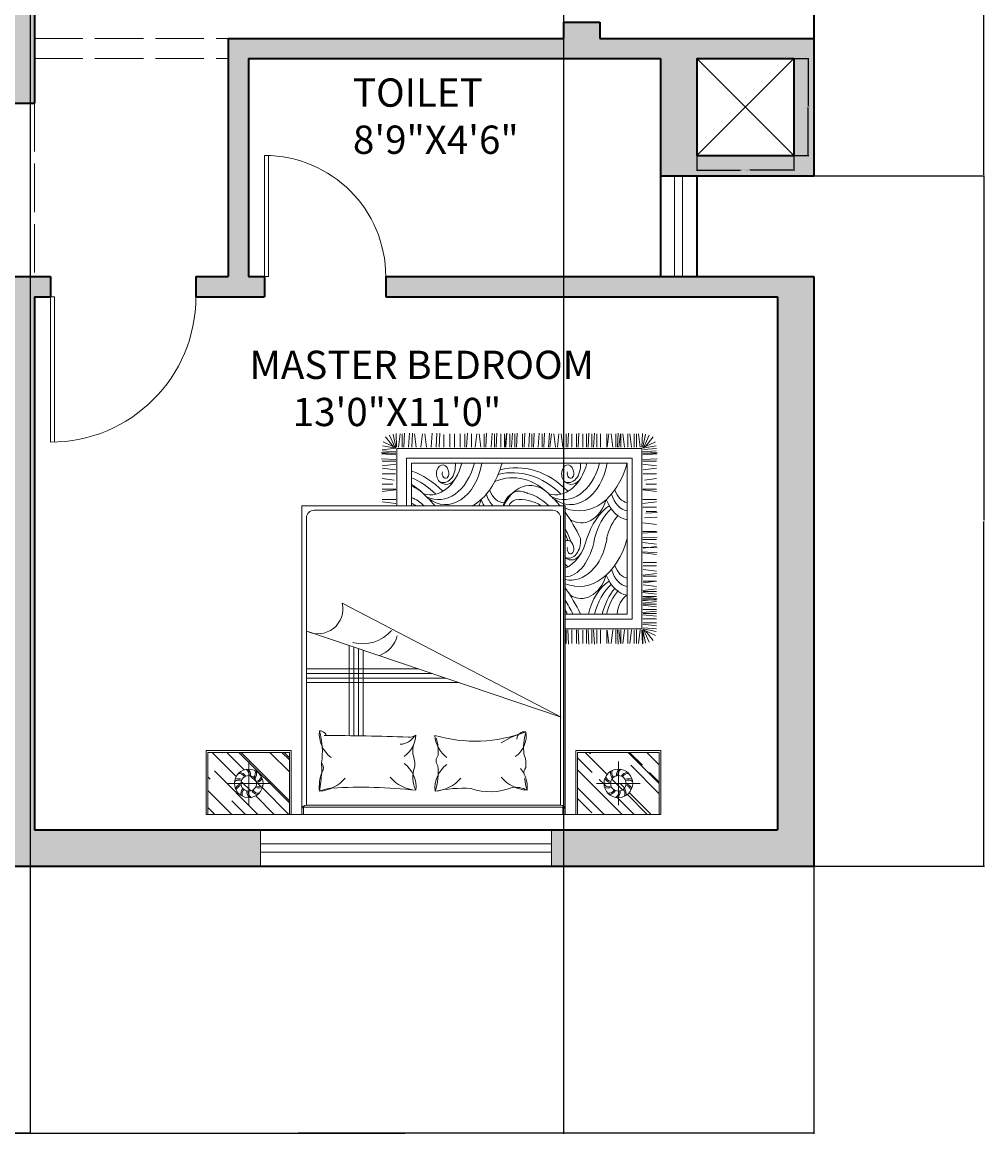
# Model space of a CAD drawing. Units: inches. Extents: x 2540 to 3167, y 3083 to 4007.
# Tile 7 of 15: x 2929 to 3167, y 3083 to 3359. Entities that reach past the tile are written whole.
import ezdxf

# ---------------------------------------------------------------- set-up
doc = ezdxf.new("R2010")
doc.units = ezdxf.units.IN
doc.linetypes.add('ACAD_ISO02W100', pattern=[15, 12, -3])
for name, color, linetype, lineweight in [('A-ANNO-DIMS', 2, 'Continuous', 18), ('A-AREA-IDEN', 7, 'Continuous', 18), ('A-DOOR', 4, 'Continuous', 18), ('A-FLOR-OPEN', 8, 'Continuous', 13), ('A-FURN', 8, 'Continuous', 13), ('A-GLAZ', 4, 'Continuous', 18)]:
    doc.layers.add(name, color=color, linetype=linetype, lineweight=lineweight)
for name, color, linetype, lineweight, true_color in [('A-WALL', 143, 'Continuous', 35, 0x7aafdf), ('A-WALL-OVHD', 143, 'ACAD_ISO02W100', 18, 0x7aafdf), ('A-WALL-PATT', 143, 'Continuous', 13, 0x7aafdf)]:
    doc.layers.add(name, color=color, linetype=linetype, lineweight=lineweight, true_color=true_color)
doc.styles.get("Standard").update_dxf_attribs({"font": 'arial.ttf'})
doc.dimstyles.get("Standard").update_dxf_attribs({"dimtxt": 0.18, "dimasz": 0.18, "dimexe": 0.18, "dimexo": 0.0625, "dimgap": 0.09, "dimtad": 0, "dimtih": 1, "dimtoh": 1, "dimdec": 4, "dimzin": 0, "dimdsep": 46, "dimtxsty": 'Standard', "dimcen": 0.09, "dimadec": 0, "dimazin": 0, "dimtfac": 1, "dimtdec": 4, "dimtofl": 0, "dimtmove": 0, "dimatfit": 3, "dimfxl": 1, "dimtolj": 1, "dimtzin": 0, "dimarcsym": 0})

# ---------------------------------------------------------------- blocks, each defined once
blk = doc.blocks.new('A$C64B41DC1')
for p, q in [((0, 2.5079), (2.9903, 2.5079)), ((0, 2.0879), (0, 2.5079)), ((0.012, 2.4618), (0.0581, 2.5079)), ((0.012, 2.3515), (0.1684, 2.5079)), ((0.012, 2.0999), (0.012, 2.5079)), ((0.0543, 2.2213), (0.3409, 2.5079)), ((0.1689, 2.4179), (0.2589, 2.5079)), ((0.3265, 2.386), (0.4484, 2.5079)), ((0.3699, 2.3332), (0.5445, 2.5079)), ((0.548, 2.5079), (0.548, 2.0999)), ((0.56, 2.5079), (0.56, 2.0879)), ((0.6301, 2.5079), (0.6301, 0.4779)), ((0.6401, 2.461), (0.6401, 2.5079)), ((0.6401, 2.5079), (2.344, 2.5079)), ((2.344, 2.5079), (2.3601, 2.5079)), ((2.344, 2.5079), (2.344, 2.461)), ((2.3601, 2.5079), (2.3601, 2.4761)), ((2.3601, 0.4779), (2.3601, 2.5079)), ((2.4303, 2.5079), (2.4303, 2.0879)), ((2.4423, 2.5079), (2.4423, 2.0999)), ((2.4423, 2.3333), (2.6169, 2.5079)), ((2.4423, 2.2145), (2.7357, 2.5079)), ((2.4423, 2.404), (2.5354, 2.4971)), ((2.705, 2.398), (2.8149, 2.5079)), ((2.7691, 2.3772), (2.8998, 2.5079)), ((2.7819, 2.3646), (2.9252, 2.5079)), ((2.9783, 2.0999), (2.9783, 2.5079)), ((2.9903, 2.0879), (2.9903, 2.5079)), ((0.2157, 2.0999), (0.548, 2.4322)), ((0.2299, 2.0999), (0.548, 2.418)), ((0.2804, 2.1597), (0.2804, 2.4481)), ((2.344, 2.461), (0.6401, 2.461)), ((0.6601, 2.4461), (1.4951, 2.4461)), ((0.6601, 2.4461), (0.6601, 0.5579)), ((1.4951, 2.4461), (0.6697, 2.4461)), ((2.3301, 2.4461), (1.4951, 2.4461)), ((2.3301, 0.5579), (2.3301, 2.4461)), ((2.7099, 2.1597), (2.7099, 2.4481)), ((0.2311, 2.2906), (0.2937, 2.3532)), ((2.6674, 2.2756), (2.7382, 2.3464)), ((2.7914, 2.1846), (2.9783, 2.3715)), ((0.012, 2.261), (0.0275, 2.2765)), ((0.1362, 2.3039), (0.4246, 2.3039)), ((0.2905, 2.2539), (0.3304, 2.2938)), ((0.3405, 2.3039), (0.3605, 2.3238)), ((2.8541, 2.3039), (2.5657, 2.3039)), ((2.5849, 2.2779), (2.6158, 2.3088)), ((2.6158, 2.3088), (2.6313, 2.3243)), ((2.7249, 2.3076), (2.7512, 2.3339)), ((2.7746, 2.0999), (2.9783, 2.3036)), ((2.9144, 2.2312), (2.9783, 2.2951)), ((0.0404, 2.0999), (0.1982, 2.2578)), ((0.1365, 2.0999), (0.251, 2.2144)), ((0.4194, 2.0999), (0.548, 2.2285)), ((2.4423, 2.1353), (2.5382, 2.2312)), ((2.4918, 2.0999), (2.6366, 2.2447)), ((0.4986, 2.0999), (0.548, 2.1493)), ((0.5127, 2.0999), (0.548, 2.1352)), ((2.7831, 2.0999), (2.8678, 2.1846)), ((2.8962, 2.0999), (2.9783, 2.182)), ((0.56, 2.0879), (0, 2.0879)), ((0.548, 2.0999), (0.012, 2.0999)), ((2.4303, 2.0879), (2.9903, 2.0879)), ((2.4423, 2.0999), (2.9783, 2.0999)), ((2.5172, 2.0999), (2.5269, 2.1096)), ((0.9415, 1.9902), (0.9415, 1.3975)), ((0.9715, 1.9906), (0.9715, 1.4076)), ((1.0015, 1.991), (1.0015, 1.4177)), ((1.0315, 1.9916), (1.0315, 1.4279)), ((2.3349, 1.8678), (0.6613, 1.3029)), ((0.8956, 1.1191), (2.3349, 1.8678)), ((1.6636, 1.6412), (0.6601, 1.6412)), ((1.5748, 1.6112), (0.6601, 1.6112)), ((2.377, 1.295), (2.3822, 1.3891)), ((2.4451, 1.295), (2.4503, 1.3891)), ((2.5105, 1.295), (2.5157, 1.3891)), ((2.5471, 1.295), (2.5524, 1.3891)), ((2.7043, 1.295), (2.7095, 1.3891)), ((2.3665, 1.295), (2.3665, 1.3839)), ((2.4032, 1.295), (2.4032, 1.3839)), ((2.4346, 1.295), (2.4346, 1.3839)), ((2.4774, 1.2957), (2.4774, 1.3837)), ((2.5, 1.295), (2.5, 1.3839)), ((2.5367, 1.295), (2.5367, 1.3839)), ((2.5681, 1.295), (2.5681, 1.3839)), ((2.5918, 1.295), (2.5918, 1.3839)), ((2.6346, 1.2957), (2.6346, 1.3837)), ((2.6362, 1.2957), (2.6467, 1.3839)), ((2.6729, 1.295), (2.6624, 1.3839)), ((2.6938, 1.295), (2.6938, 1.3839)), ((2.7127, 1.2957), (2.7232, 1.3839)), ((2.7253, 1.295), (2.7253, 1.3839)), ((2.7494, 1.295), (2.7389, 1.3839)), ((2.7718, 1.295), (2.7718, 1.3839)), ((2.7959, 1.295), (2.7854, 1.3839)), ((2.8146, 1.2957), (2.8146, 1.3837)), ((2.8146, 1.2957), (2.8146, 1.3837)), ((2.8282, 1.295), (2.8282, 1.3839)), ((2.8282, 1.295), (2.8282, 1.3839)), ((2.8523, 1.295), (2.8418, 1.3839)), ((2.8523, 1.295), (2.8418, 1.3839)), ((2.8653, 1.2966), (2.8688, 1.3861)), ((2.8711, 1.2957), (2.8711, 1.3837)), ((2.8711, 1.2957), (2.8875, 1.3822)), ((2.8713, 1.2927), (2.954, 1.3315)), ((2.8765, 1.2958), (2.9132, 1.3758)), ((2.8893, 1.3011), (2.9394, 1.3636)), ((2.3601, 1.2873), (2.8639, 1.2873)), ((2.8639, 1.2873), (2.8639, 0.1018)), ((2.8716, 1.2565), (2.9605, 1.2669)), ((2.8717, 1.2884), (2.9588, 1.3058)), ((2.8723, 1.2489), (2.9603, 1.2489)), ((2.8744, 1.2817), (2.9603, 1.2869)), ((2.3601, 1.2233), (2.7999, 1.2233)), ((2.3601, 1.1913), (2.7679, 1.1912)), ((2.7679, 1.1912), (2.7679, 0.1978)), ((2.7999, 1.2233), (2.7999, 0.1658)), ((2.8716, 1.2212), (2.9605, 1.2212)), ((2.8716, 1.1947), (2.9605, 1.2052)), ((2.8716, 1.181), (2.9605, 1.1705)), ((2.8723, 1.1872), (2.9603, 1.1872)), ((2.8716, 1.1595), (2.9605, 1.1595)), ((2.8716, 1.133), (2.9605, 1.1435)), ((2.8716, 1.1193), (2.9605, 1.1088)), ((2.8716, 1.1035), (2.9605, 1.093)), ((2.8716, 1.0965), (2.9605, 1.0965)), ((2.8723, 1.1255), (2.9603, 1.1255)), ((2.8716, 1.086), (2.9657, 1.0913)), ((2.8716, 1.0756), (2.9605, 1.0756)), ((2.8716, 1.0491), (2.9605, 1.0596)), ((2.8716, 1.0354), (2.9605, 1.0249)), ((2.8723, 1.0858), (2.9605, 1.0753)), ((2.8723, 1.0416), (2.9603, 1.0416)), ((2.8723, 0.9987), (2.9605, 1.0092)), ((2.8723, 0.985), (2.9605, 0.9745)), ((2.8723, 0.9735), (2.9603, 0.9735)), ((2.8716, 0.9346), (2.9605, 0.9241)), ((2.8723, 0.9408), (2.9603, 0.9408)), ((2.8723, 0.8979), (2.9605, 0.9084)), ((2.8723, 0.8726), (2.9603, 0.8726)), ((2.8723, 0.8505), (2.9603, 0.8505)), ((2.8716, 0.7885), (2.9605, 0.799)), ((2.8716, 0.7818), (2.9657, 0.787)), ((2.8716, 0.7503), (2.9657, 0.7556)), ((2.8716, 0.7204), (2.9605, 0.7309)), ((2.8723, 0.7571), (2.9605, 0.7466)), ((2.8716, 0.6995), (2.9605, 0.6995)), ((2.8716, 0.689), (2.9657, 0.6838)), ((2.8716, 0.6576), (2.9657, 0.6523)), ((2.8716, 0.6471), (2.9605, 0.6471)), ((2.8716, 0.5903), (2.9605, 0.6007)), ((2.882, 0.5582), (2.9657, 0.5536)), ((2.8909, 0.5263), (2.9657, 0.5222)), ((2.8928, 0.5169), (2.9605, 0.5169)), ((0.6301, 0.4779), (2.3601, 0.4779)), ((0.7101, 0.5079), (2.2801, 0.5079)), ((1.2465, 0.4625), (1.1576, 0.452)), ((1.2542, 0.1018), (1.2542, 0.4779)), ((1.3182, 0.1658), (1.3182, 0.4779)), ((1.3502, 0.1978), (1.3502, 0.4779)), ((2.8716, 0.4877), (2.9603, 0.4877)), ((2.8716, 0.4625), (2.9605, 0.452)), ((1.2465, 0.3746), (1.1576, 0.3851)), ((1.2465, 0.4365), (1.1577, 0.4365)), ((1.2465, 0.3684), (1.1577, 0.3684)), ((2.8716, 0.4365), (2.9603, 0.4365)), ((2.8716, 0.3746), (2.9605, 0.3851)), ((2.8716, 0.3684), (2.9603, 0.3684)), ((1.2355, 0.3092), (1.1576, 0.3)), ((1.2285, 0.3357), (1.1577, 0.3357)), ((2.8826, 0.3092), (2.9605, 0.3)), ((2.8896, 0.3357), (2.9603, 0.3357)), ((1.2457, 0.2423), (1.1576, 0.2319)), ((1.2457, 0.2676), (1.1577, 0.2676)), ((2.8723, 0.2676), (2.9603, 0.2676)), ((2.8723, 0.2423), (2.9605, 0.2319)), ((1.2465, 0.1742), (1.1524, 0.169)), ((1.2465, 0.2057), (1.1576, 0.2161)), ((1.2465, 0.1847), (1.1576, 0.1847)), ((2.7999, 0.1658), (1.3182, 0.1658)), ((2.7679, 0.1978), (1.3502, 0.1978)), ((2.8716, 0.2057), (2.9605, 0.2161)), ((2.8716, 0.1847), (2.9605, 0.1847)), ((2.8716, 0.1742), (2.9657, 0.169)), ((1.2465, 0.1428), (1.1524, 0.1376)), ((1.2465, 0.1334), (1.1524, 0.1281)), ((1.2465, 0.1323), (1.1576, 0.1323)), ((1.2465, 0.1323), (1.1576, 0.1323)), ((1.2465, 0.1), (1.1576, 0.1105)), ((1.2465, 0.1229), (1.1588, 0.1168)), ((1.2464, 0.1007), (1.1592, 0.0833)), ((1.2468, 0.0964), (1.1641, 0.0576)), ((1.2288, 0.088), (1.1787, 0.0255)), ((1.2415, 0.0933), (1.2049, 0.0133)), ((1.247, 0.0934), (1.2306, 0.0069)), ((1.2527, 0.0925), (1.2493, 0.003)), ((2.8639, 0.1018), (1.2542, 0.1018)), ((1.2658, 0.0941), (1.2762, 0.0052)), ((1.2899, 0.0941), (1.2899, 0.0052)), ((1.2999, 0.0941), (1.3051, 0)), ((1.3313, 0.0941), (1.3365, 0)), ((1.3523, 0.0941), (1.3575, 0)), ((1.3804, 0.0941), (1.3699, 0.0052)), ((1.4119, 0.0934), (1.4223, 0.0052)), ((1.4485, 0.0941), (1.438, 0.0052)), ((1.48, 0.0941), (1.4852, 0)), ((1.5114, 0.0941), (1.5166, 0)), ((1.5323, 0.0941), (1.5376, 0)), ((1.5638, 0.0941), (1.5638, 0.0105)), ((1.6021, 0.0941), (1.6021, 0.0052)), ((1.6336, 0.0941), (1.6336, 0.0052)), ((1.6702, 0.0941), (1.6702, 0.0052)), ((1.7017, 0.0941), (1.7017, 0.0052)), ((1.7122, 0.0941), (1.7174, 0)), ((1.7445, 0.0934), (1.7445, 0.0054)), ((1.7698, 0.0934), (1.7803, 0.0052)), ((1.8065, 0.0941), (1.796, 0.0052)), ((1.8274, 0.0941), (1.8274, 0.0052)), ((1.8379, 0.0941), (1.8431, 0)), ((1.8746, 0.0941), (1.8798, 0)), ((1.8955, 0.0941), (1.8955, 0.0052)), ((1.906, 0.0941), (1.9113, 0)), ((1.9384, 0.0934), (1.9384, 0.0054)), ((1.9609, 0.0941), (1.9609, 0.0052)), ((1.9636, 0.0934), (1.9741, 0.0052)), ((1.9714, 0.0941), (1.9766, 0)), ((1.9976, 0.0941), (1.9976, 0.0052)), ((2.0081, 0.0941), (2.0133, 0)), ((2.029, 0.0941), (2.029, 0.0052)), ((2.0395, 0.0941), (2.0447, 0)), ((2.0797, 0.0941), (2.0797, 0.0052)), ((2.0902, 0.0941), (2.0954, 0)), ((2.1216, 0.0941), (2.1269, 0)), ((2.1412, 0.0941), (2.1412, 0.0052)), ((2.1517, 0.0941), (2.1569, 0)), ((2.1831, 0.0941), (2.1884, 0)), ((2.2093, 0.0941), (2.2093, 0.0052)), ((2.2198, 0.0941), (2.225, 0)), ((2.2512, 0.0941), (2.2565, 0)), ((2.2603, 0.0934), (2.2707, 0.0052)), ((2.2969, 0.0941), (2.2864, 0.0052)), ((2.3089, 0.0934), (2.3193, 0.0052)), ((2.3455, 0.0941), (2.3351, 0.0052)), ((2.3665, 0.0941), (2.3665, 0.0052)), ((2.377, 0.0941), (2.3822, 0)), ((2.4032, 0.0941), (2.4032, 0.0052)), ((2.4346, 0.0941), (2.4346, 0.0052)), ((2.4451, 0.0941), (2.4503, 0)), ((2.4774, 0.0934), (2.4774, 0.0054)), ((2.5, 0.0941), (2.5, 0.0052)), ((2.5105, 0.0941), (2.5157, 0)), ((2.5367, 0.0941), (2.5367, 0.0052)), ((2.5471, 0.0941), (2.5524, 0)), ((2.5681, 0.0941), (2.5681, 0.0052)), ((2.5918, 0.0941), (2.5918, 0.0052)), ((2.6346, 0.0934), (2.6346, 0.0054)), ((2.6362, 0.0934), (2.6467, 0.0052)), ((2.6729, 0.0941), (2.6624, 0.0052)), ((2.6938, 0.0941), (2.6938, 0.0052)), ((2.7043, 0.0941), (2.7095, 0)), ((2.7127, 0.0934), (2.7232, 0.0052)), ((2.7253, 0.0941), (2.7253, 0.0052)), ((2.7494, 0.0941), (2.7389, 0.0052)), ((2.7718, 0.0941), (2.7718, 0.0052)), ((2.7959, 0.0941), (2.7854, 0.0052)), ((2.8146, 0.0934), (2.8146, 0.0054)), ((2.8282, 0.0941), (2.8282, 0.0052)), ((2.8523, 0.0941), (2.8418, 0.0052)), ((2.8653, 0.0925), (2.8688, 0.003)), ((2.8711, 0.0934), (2.8875, 0.0069)), ((2.8713, 0.0964), (2.954, 0.0576)), ((2.8716, 0.1428), (2.9657, 0.1376)), ((2.8716, 0.1334), (2.9657, 0.1281)), ((2.8716, 0.1323), (2.9605, 0.1323)), ((2.8716, 0.1229), (2.9593, 0.1168)), ((2.8717, 0.1007), (2.9588, 0.0833)), ((2.8744, 0.1074), (2.9603, 0.1022)), ((2.8765, 0.0933), (2.9132, 0.0133)), ((2.8893, 0.088), (2.9394, 0.0255))]:
    blk.add_line(p, q)
at = {"ltscale": 10}
for p, q in [((1.4859, 1.5812), (0.6601, 1.5812)), ((1.397, 1.5512), (0.6601, 1.5512))]:
    blk.add_line(p, q, dxfattribs=at)
for centre, radius in [((0.2804, 2.3039), 0.0942), ((0.2804, 2.3039), 0.051), ((2.7099, 2.3039), 0.0942), ((2.7099, 2.3039), 0.051)]:
    blk.add_circle(centre, radius)
for centre, radius, start, end in [((0.6601, 2.4761), 0.03, 180, 270), ((2.3301, 2.4761), 0.03, 270, 0), ((0.2417, 2.3614), 0.0462, 196.30017, 256.53802), ((0.2887, 2.3745), 0.0605, 172.17003, 218.48975), ((0.2828, 2.3731), 0.0462, 160.30017, 220.53802), ((0.3286, 2.3561), 0.0605, 136.17003, 182.48975), ((0.3231, 2.3585), 0.0462, 124.30017, 184.53802), ((0.3501, 2.3178), 0.0605, 100.17003, 146.48975), ((0.347, 2.323), 0.0462, 88.30017, 148.53802), ((1.0526, 2.3302), 0.3085, 175.30484, 198.69419), ((-0.8702, 2.0941), 1.6364, 4.80985, 9.18918), ((0.8579, 2.6278), 0.2948, 247.51785, 264.26696), ((0.728, 2.111), 0.245, 40.4189, 85.9871), ((1.0164, 5.7096), 3.3803, 266.81337, 276.16021), ((1.3963, 2.1044), 0.245, 94.0129, 139.5811), ((1.1858, 2.3288), 0.1943, 306.5711, 5.88998), ((1.5348, 2.2652), 0.1767, 151.77364, 201.69827), ((1.6986, 2.3355), 0.1943, 174.11002, 233.4289), ((1.1481, 2.2311), 0.3783, 353.49469, 19.18669), ((1.6871, 3.192), 0.8561, 257.74383, 273.62843), ((1.4882, 2.111), 0.245, 40.4189, 85.9871), ((1.8674, 1.9709), 0.3878, 68.20259, 108.9817), ((2.1269, 2.1044), 0.245, 94.0129, 139.5811), ((2.0342, 2.4856), 0.1563, 261.59582, 298.90918), ((1.9165, 2.3288), 0.1943, 333.73715, 5.88998), ((2.6058, 2.2028), 0.517, 163.60457, 172.3273), ((2.6433, 2.323), 0.0462, 31.46198, 91.69983), ((2.6402, 2.3178), 0.0605, 33.51025, 79.82997), ((2.6672, 2.3585), 0.0462, 355.46198, 55.69983), ((2.6617, 2.3561), 0.0605, 357.51025, 43.82997), ((2.7075, 2.3731), 0.0462, 319.46198, 19.69983), ((2.7016, 2.3745), 0.0605, 321.51025, 7.82997), ((2.7486, 2.3614), 0.0462, 283.46198, 343.69983), ((0.2153, 2.3276), 0.0462, 232.30017, 292.53802), ((0.2158, 2.3336), 0.0605, 244.17003, 290.48975), ((0.2457, 2.3659), 0.0605, 208.17003, 254.48975), ((0.272, 2.2333), 0.0605, 352.17003, 38.48975), ((0.3449, 2.2742), 0.0605, 64.17003, 110.48975), ((0.3455, 2.2802), 0.0462, 52.30017, 112.53802), ((0.3191, 2.2464), 0.0462, 16.30017, 76.53802), ((0.3151, 2.2419), 0.0605, 28.17003, 74.48975), ((2.6448, 2.2802), 0.0462, 67.46198, 127.69983), ((2.6454, 2.2742), 0.0605, 69.51025, 115.82997), ((2.6752, 2.2419), 0.0605, 105.51025, 151.82997), ((2.6712, 2.2464), 0.0462, 103.46198, 163.69983), ((2.7182, 2.2333), 0.0605, 141.51025, 187.82997), ((2.7744, 2.3336), 0.0605, 249.51025, 295.82997), ((2.775, 2.3276), 0.0462, 247.46198, 307.69983), ((2.7446, 2.3659), 0.0605, 285.51025, 331.82997), ((0.2138, 2.2848), 0.0462, 268.30017, 328.53802), ((0.2107, 2.29), 0.0605, 280.17003, 326.48975), ((0.2377, 2.2493), 0.0462, 304.30017, 4.53802), ((0.2322, 2.2517), 0.0605, 316.17003, 2.48975), ((0.2779, 2.2347), 0.0462, 340.30017, 40.53802), ((0.7274, 2.2013), 0.0446, 314.4736, 42.17134), ((-1.6008, 2.277), 2.3618, 357.39054, 358.88764), ((1.204, 2.1778), 0.1681, 337.01697, 7.53676), ((1.9165, 2.3288), 0.1943, 320.94042, 333.73715), ((2.1347, 2.2313), 0.0459, 165.35061, 223.26844), ((1.9346, 2.1778), 0.1681, 337.01697, 7.53676), ((2.7123, 2.2347), 0.0462, 139.46198, 199.69983), ((2.7581, 2.2517), 0.0605, 177.51025, 223.82997), ((2.7526, 2.2493), 0.0462, 175.46198, 235.69983), ((2.7796, 2.29), 0.0605, 213.51025, 259.82997), ((2.7765, 2.2848), 0.0462, 211.46198, 271.69983), ((0.9385, 1.978), 0.1943, 126.5711, 185.88998), ((0.2688, 2.0945), 0.4956, 344.0243, 8.70709), ((1.1858, 1.9714), 0.1943, 4.31813, 53.4289), ((1.7059, 1.9714), 0.204, 127.11975, 175.09005), ((1.5671, 2.1546), 0.0547, 142.08329, 220.902), ((1.9394, 1.991), 0.1651, 351.26213, 55.75721), ((1.2687, 1.9248), 0.1223, 33.62799, 86.47438), ((1.5415, 2.0969), 0.1834, 175.22328, 196.23004), ((1.1965, 2.0983), 0.3299, 343.79543, 3.55541), ((2.4617, 2.0719), 0.3745, 173.82958, 196.4356), ((0.7417, 2.0149), 0.057, 273.47085, 328.54118), ((0.7246, 18.8439), 16.8552, 270.17399, 272.05214), ((1.3401, 1.9404), 0.0603, 49.09906, 101.37023), ((1.7676, 1.0629), 0.9631, 69.65065, 105.96307), ((2.2748, 2.5795), 0.6373, 238.34989, 254.31375), ((2.0911, 2.0123), 0.0478, 179.77267, 283.80184), ((0.728, 2.2025), 0.245, 274.0129, 278.34166), ((1.0747, 1.2871), 0.1871, 14.1863, 69.12121), ((0.7347, 1.1553), 0.1649, 347.31088, 116.44537), ((1.0274, 1.1334), 0.2527, 40.62904, 104.37123), ((0.7101, 0.5579), 0.05, 180, 270), ((2.2801, 0.5579), 0.05, 270, 0)]:
    blk.add_arc(centre, radius, start, end)
for centre, major_axis, ratio, start_param, end_param in [((1.9938, 1.6262), (0, -0.7531), 0.68, 0.797284, 0.954936), ((2.0643, 1.466), (0, -0.5322), 0.68, 7.239912, 7.311536), ((1.9052, 1.7397), (0, -0.9842), 0.68, 0.74745, 0.979724), ((2.7455, 1.3081), (0, 0.3614), 0.68, 1.900046, 2.742661), ((2.7868, 1.3081), (0, 0.3614), 0.68, 1.900046, 2.614747), ((2.8372, 1.3081), (0, 0.3614), 0.68, 1.900046, 2.479658), ((2.8607, 1.3211), (0, 0.3614), 0.68, 1.938265, 2.479658), ((2.8057, 1.2079), (0, -0.1524), 0.68, 4.821745, 5.895886), ((2.4665, 0.8216), (0, -0.2664), 0.68, 2.006169, 3.565187), ((2.4513, 0.5069), (0, 0.502), 0.68, 5.095327, 6.553458), ((2.7862, 0.8069), (0, -0.2615), 0.68, 3.244645, 4.205018), ((2.396, 0.6032), (0, 0.3641), 0.68, -1.3172, 0.145284), ((2.7784, 0.8289), (0, -0.1802), 0.68, 3.227058, 4.318474), ((2.7821, 0.7971), (0, -0.1589), 0.68, 3.272942, 4.229533), ((2.3507, 0.5642), (0.0073, 0.3819), 0.56205, -1.21172, -0.009991), ((2.2964, 0.5771), (0, -0.3263), 0.68, 1.938944, 2.850232), ((2.0403, 1.6015), (0, -0.8763), 0.68, 6.849801, 6.887077), ((2.4005, 0.7132), (0, -0.1214), 0.68, 2.284368, 3.652258), ((2.3834, 0.7081), (0, 0.1147), 0.68, 4.593909, 6.585576), ((2.3774, 0.7653), (0, -0.0593), 0.68, 5.841311, 7.755362), ((2.3961, 0.7628), (0, -0.0317), 0.68, 1.462497, 5.046281), ((1.9938, 1.1295), (-0.0678, 0.7439), 0.610498, 3.917146, 4.063997), ((2.0643, 0.9693), (0, -0.5322), 0.68, 7.239912, 7.336618), ((1.9052, 1.243), (0, -0.9842), 0.68, 0.74745, 0.979724), ((2.7455, 0.8114), (-0.0599, 0.3735), 0.695517, 1.775813, 2.548612), ((2.7868, 0.8114), (0, 0.3614), 0.68, 1.900046, 2.614747), ((2.8607, 0.8243), (0, 0.3614), 0.68, 1.938265, 2.479658), ((2.4665, 0.3249), (0, -0.2664), 0.68, 2.006169, 3.565187), ((2.4513, 0.0102), (0, 0.502), 0.68, 5.095327, 6.553458), ((2.7862, 0.3102), (0, -0.2615), 0.68, 3.244645, 4.205018), ((2.7784, 0.3322), (0, -0.1802), 0.68, 3.227058, 4.318474), ((1.242, 0.9693), (0, -0.5322), 0.68, 6.586764, 6.677612), ((1.1714, 1.1295), (-0.1157, 0.7241), 0.59432, 3.291697, 3.50733), ((1.0828, 1.243), (0, -0.9842), 0.68, 0.565948, 0.680366), ((1.5283, 0.0674), (0, -0.3703), 0.68, 1.930561, 3.464283), ((1.5736, 0.1065), (0, 0.3641), 0.68, -1.3172, 0.476403), ((1.6289, 0.0102), (0, 0.502), 0.68, 6.655152, 6.661293), ((1.6289, 0.0102), (0, 0.502), 0.68, 5.095327, 5.911219), ((1.6442, 0.3249), (0, -0.2664), 0.68, 2.006169, 2.182797), ((1.9638, 0.3102), (0, -0.2615), 0.68, 4.015924, 4.205018), ((1.956, 0.3322), (0, -0.1802), 0.68, 3.770744, 4.318474), ((1.9597, 0.3004), (0, -0.1589), 0.68, 3.14258, 4.229533), ((2.0606, 0.5616), (0, -0.1803), 0.68, 5.194792, 5.929328), ((2.0606, 0.5616), (0, -0.1803), 0.68, 5.194792, 6.723255), ((2.1315, 0.6603), (0, -0.3155), 0.68, 5.328638, 6.949396), ((2.0549, 0.5656), (0, -0.1303), 0.68, 5.450951, 6.054641), ((2.0643, 0.9693), (0, -0.5322), 0.68, 6.20013, 6.677612), ((1.9938, 1.1295), (-0.0678, 0.7439), 0.610498, 3.199135, 3.592282), ((1.9052, 1.243), (0, -0.9842), 0.68, 0.565948, 0.680366), ((2.3507, 0.0674), (0, -0.3703), 0.68, 1.930561, 3.464283), ((2.396, 0.1065), (0, 0.3641), 0.68, -1.3172, 0.476403), ((2.4513, 0.0102), (0, 0.502), 0.68, 6.655152, 6.661293), ((2.7821, 0.3004), (0, -0.1589), 0.68, 3.272942, 4.229533), ((1.1933, 0.9181), (0, -0.624), 0.68, 0.378672, 0.625379), ((1.3091, 0.6603), (0, -0.3155), 0.68, 6.475719, 6.949396), ((1.1911, 1.1066), (0, 0.8458), 0.68, 3.421828, 3.728616), ((1.2179, 1.1047), (0, -0.8763), 0.68, 6.507006, 6.887077), ((1.474, 0.0804), (0, -0.3263), 0.68, 1.938944, 3.339184), ((2.0157, 0.9181), (0, -0.624), 0.68, -0.280078, 0.625379), ((2.0135, 1.1066), (0, 0.8458), 0.68, 2.978727, 3.728616), ((2.0403, 1.1047), (0, -0.8763), 0.68, 6.099302, 6.887077), ((2.2964, 0.0804), (0, -0.3263), 0.68, 1.938944, 3.339184), ((1.555, 0.2685), (0, -0.0593), 0.68, 3.732151, 7.755362), ((1.5781, 0.2165), (0, -0.1214), 0.68, 2.284368, 3.726131), ((1.561, 0.2114), (0, 0.1147), 0.68, 4.593909, 6.647252), ((1.5737, 0.2661), (0, -0.0317), 0.68, 1.462497, 5.046281), ((2.3774, 0.2685), (0, -0.0593), 0.68, 3.732151, 7.755362), ((2.4005, 0.2165), (0, -0.1214), 0.68, 2.284368, 3.726131), ((2.3834, 0.2114), (0, 0.1147), 0.68, 4.593909, 6.647252), ((2.3961, 0.2661), (0, -0.0317), 0.68, 1.462497, 5.046281)]:
    blk.add_ellipse(centre, major_axis=major_axis, ratio=ratio, start_param=start_param, end_param=end_param)
blk = doc.blocks.new('DOOR-SWING-36IN')
for p, q in [((36, 0), (0, 0)), ((36, 1), (0.01, 1)), ((36, 1), (36, 0))]:
    blk.add_line(p, q)
blk.add_arc((36, 0), 36, 90, 180)
blk = doc.blocks.new('DOOR-SWING-30IN')
for p, q in [((0, 0), (0, 30)), ((1, 0), (1, 29.98)), ((0, 0), (1, 0))]:
    blk.add_line(p, q)
blk.add_arc((0, 0), 30, 0, 90)
blk = doc.blocks.new('WIN-72IN')
for p, q in [((9, 72), (0, 72)), ((3.5, 0), (3.5, 72)), ((5.5, 0), (5.5, 72)), ((9, 0), (0, 0))]:
    blk.add_line(p, q)
blk = doc.blocks.new('OPENING-CROSS-24IN')
for p, q in [((24, 24), (0, 0)), ((0, 24), (24, 0))]:
    blk.add_line(p, q)
blk = doc.blocks.new('*D41')
at = {"layer": 'A-ANNO-DIMS', "color": 0, "lineweight": -2, "transparency": 16777216}
for p, q in [((3095.51, 3325.65), (3095.51, 3321.93)), ((3119.51, 3325.65), (3119.51, 3321.93)), ((3095.69, 3322.11), (3106.37, 3322.11)), ((3119.33, 3322.11), (3108.65, 3322.11))]:
    blk.add_line(p, q, dxfattribs=at)
at = {"layer": 'A-ANNO-DIMS', "color": 0, "transparency": 16777216}
for points in [[(3095.69, 3322.14), (3095.69, 3322.08), (3095.51, 3322.11)], [(3119.33, 3322.14), (3119.33, 3322.08), (3119.51, 3322.11)]]:
    blk.add_solid(points, dxfattribs=at)
at = {"layer": 'Defpoints', "color": 0, "transparency": 16777216}
for p in [(3095.51, 3325.71), (3119.51, 3325.71), (3119.51, 3322.11)]:
    blk.add_point(p, dxfattribs=at)
at = {"layer": 'A-ANNO-DIMS', "color": 0, "transparency": 16777216, "insert": (3107.51, 3322.11), "char_height": 0.18, "attachment_point": 5}
blk.add_mtext('\\A1;OPENING 24 TYP.', dxfattribs=at)
blk = doc.blocks.new('*D42')
at = {"layer": 'A-ANNO-DIMS', "color": 0, "lineweight": -2, "transparency": 16777216}
for p, q in [((3119.57, 3349.71), (3123.29, 3349.71)), ((3123.11, 3349.53), (3123.11, 3337.89)), ((3123.11, 3325.89), (3123.11, 3337.53)), ((3119.57, 3325.71), (3123.29, 3325.71))]:
    blk.add_line(p, q, dxfattribs=at)
at = {"layer": 'A-ANNO-DIMS', "color": 0, "transparency": 16777216}
for points in [[(3123.08, 3349.53), (3123.14, 3349.53), (3123.11, 3349.71)], [(3123.08, 3325.89), (3123.14, 3325.89), (3123.11, 3325.71)]]:
    blk.add_solid(points, dxfattribs=at)
at = {"layer": 'Defpoints', "color": 0, "transparency": 16777216}
for p in [(3119.51, 3349.71), (3123.11, 3349.71), (3119.51, 3325.71)]:
    blk.add_point(p, dxfattribs=at)
at = {"layer": 'A-ANNO-DIMS', "color": 0, "transparency": 16777216, "insert": (3123.11, 3337.71), "char_height": 0.18, "attachment_point": 5}
blk.add_mtext('\\A1;24 TYP.', dxfattribs=at)
blk = doc.blocks.new('*D47')
at = {"layer": 'A-ANNO-DIMS', "color": 0, "lineweight": -2, "transparency": 16777216}
for p, q in [((3124.51, 3149.65), (3124.51, 3083.43)), ((2922.51, 3125.65), (2922.51, 3083.43)), ((2922.69, 3083.61), (3023.22, 3083.61)), ((3124.33, 3083.61), (3023.8, 3083.61))]:
    blk.add_line(p, q, dxfattribs=at)
at = {"layer": 'A-ANNO-DIMS', "color": 0, "transparency": 16777216}
for points in [[(2922.69, 3083.64), (2922.69, 3083.58), (2922.51, 3083.61)], [(3124.33, 3083.64), (3124.33, 3083.58), (3124.51, 3083.61)]]:
    blk.add_solid(points, dxfattribs=at)
at = {"layer": 'Defpoints', "color": 0, "transparency": 16777216}
for p in [(3124.51, 3149.71), (2922.51, 3125.71), (3124.51, 3083.61)]:
    blk.add_point(p, dxfattribs=at)
at = {"layer": 'A-ANNO-DIMS', "color": 0, "transparency": 16777216, "insert": (3023.51, 3083.61), "char_height": 0.18, "attachment_point": 5}
blk.add_mtext('\\A1;202', dxfattribs=at)
blk = doc.blocks.new('*D52')
at = {"layer": 'A-ANNO-DIMS', "color": 0, "lineweight": -2, "transparency": 16777216}
for p, q in [((3124.57, 3462.71), (3166.79, 3462.71)), ((3166.61, 3462.53), (3166.61, 3391.89)), ((3166.61, 3320.89), (3166.61, 3391.53)), ((3124.57, 3320.71), (3166.79, 3320.71))]:
    blk.add_line(p, q, dxfattribs=at)
at = {"layer": 'A-ANNO-DIMS', "color": 0, "transparency": 16777216}
for points in [[(3166.58, 3462.53), (3166.64, 3462.53), (3166.61, 3462.71)], [(3166.58, 3320.89), (3166.64, 3320.89), (3166.61, 3320.71)]]:
    blk.add_solid(points, dxfattribs=at)
at = {"layer": 'Defpoints', "color": 0, "transparency": 16777216}
for p in [(3124.51, 3462.71), (3124.51, 3320.71), (3166.61, 3320.71)]:
    blk.add_point(p, dxfattribs=at)
at = {"layer": 'A-ANNO-DIMS', "color": 0, "transparency": 16777216, "insert": (3166.61, 3391.71), "char_height": 0.18, "attachment_point": 5}
blk.add_mtext('\\A1;142', dxfattribs=at)
blk = doc.blocks.new('*D53')
at = {"layer": 'A-ANNO-DIMS', "color": 0, "lineweight": -2, "transparency": 16777216}
for p, q in [((3124.57, 3320.71), (3166.79, 3320.71)), ((3166.61, 3320.53), (3166.61, 3235.39)), ((3166.61, 3149.89), (3166.61, 3235.03)), ((3124.57, 3149.71), (3166.79, 3149.71))]:
    blk.add_line(p, q, dxfattribs=at)
at = {"layer": 'A-ANNO-DIMS', "color": 0, "transparency": 16777216}
for points in [[(3166.58, 3320.53), (3166.64, 3320.53), (3166.61, 3320.71)], [(3166.58, 3149.89), (3166.64, 3149.89), (3166.61, 3149.71)]]:
    blk.add_solid(points, dxfattribs=at)
at = {"layer": 'Defpoints', "color": 0, "transparency": 16777216}
for p in [(3124.51, 3320.71), (3124.51, 3149.71), (3166.61, 3149.71)]:
    blk.add_point(p, dxfattribs=at)
at = {"layer": 'A-ANNO-DIMS', "color": 0, "transparency": 16777216, "insert": (3166.61, 3235.21), "char_height": 0.18, "attachment_point": 5}
blk.add_mtext('\\A1;171', dxfattribs=at)
blk = doc.blocks.new('*D54')
at = {"layer": 'A-ANNO-DIMS', "color": 0, "lineweight": -2, "transparency": 16777216}
for p, q in [((2930.51, 3543.65), (2930.51, 3083.43)), ((3062.51, 3543.65), (3062.51, 3083.43)), ((2930.69, 3083.61), (2996.23, 3083.61)), ((3062.33, 3083.61), (2996.79, 3083.61))]:
    blk.add_line(p, q, dxfattribs=at)
at = {"layer": 'A-ANNO-DIMS', "color": 0, "transparency": 16777216}
for points in [[(2930.69, 3083.64), (2930.69, 3083.58), (2930.51, 3083.61)], [(3062.33, 3083.64), (3062.33, 3083.58), (3062.51, 3083.61)]]:
    blk.add_solid(points, dxfattribs=at)
at = {"layer": 'Defpoints', "color": 0, "transparency": 16777216}
for p in [(2930.51, 3543.71), (3062.51, 3543.71), (3062.51, 3083.61)]:
    blk.add_point(p, dxfattribs=at)
at = {"layer": 'A-ANNO-DIMS', "color": 0, "transparency": 16777216, "insert": (2996.51, 3083.61), "char_height": 0.18, "attachment_point": 5}
blk.add_mtext('\\A1;132', dxfattribs=at)
blk = doc.blocks.new('*D55')
at = {"layer": 'A-ANNO-DIMS', "color": 0, "lineweight": -2, "transparency": 16777216}
for p, q in [((2868.51, 3564.65), (2868.51, 3083.43)), ((2930.51, 3543.65), (2930.51, 3083.43)), ((2868.69, 3083.61), (2899.29, 3083.61)), ((2930.33, 3083.61), (2899.73, 3083.61))]:
    blk.add_line(p, q, dxfattribs=at)
at = {"layer": 'A-ANNO-DIMS', "color": 0, "transparency": 16777216}
for points in [[(2868.69, 3083.64), (2868.69, 3083.58), (2868.51, 3083.61)], [(2930.33, 3083.64), (2930.33, 3083.58), (2930.51, 3083.61)]]:
    blk.add_solid(points, dxfattribs=at)
at = {"layer": 'Defpoints', "color": 0, "transparency": 16777216}
for p in [(2868.51, 3564.71), (2930.51, 3543.71), (2930.51, 3083.61)]:
    blk.add_point(p, dxfattribs=at)
at = {"layer": 'A-ANNO-DIMS', "color": 0, "transparency": 16777216, "insert": (2899.51, 3083.61), "char_height": 0.18, "attachment_point": 5}
blk.add_mtext('\\A1;62', dxfattribs=at)

msp = doc.modelspace()

# ---------------------------------------------------------------- hatches: boundary and pattern name
at = {"layer": 'A-WALL-PATT'}
h = msp.add_hatch(color=256, dxfattribs=at)
h.dxf.hatch_style = 1
h.paths.add_polyline_path([(2805.51, 3803.71), (2800.51, 3803.71), (2800.51, 3799.71), (2621.51, 3799.71), (2621.51, 3823.71), (2612.51, 3823.71), (2612.51, 3794.71), (2636.51, 3794.71), (2636.51, 3782.71), (2645.51, 3782.71), (2645.51, 3794.71), (2805.51, 3794.71)])
h.paths.add_polyline_path([(2810.51, 3564.71), (2868.51, 3564.71), (2868.51, 3627.71), (2872.51, 3627.71), (2872.51, 3636.71), (2864.51, 3636.71), (2864.51, 3674.71), (2797.51, 3674.71), (2797.51, 3669.71), (2801.51, 3669.71), (2801.51, 3628.63), (2806.51, 3628.63), (2806.51, 3669.71), (2859.51, 3669.71), (2859.51, 3573.71), (2806.51, 3573.71), (2806.51, 3598.63), (2801.51, 3598.63), (2801.51, 3549.71), (2645.51, 3549.71), (2645.51, 3573.71), (2636.51, 3573.71), (2636.51, 3516.71), (2645.51, 3516.71), (2645.51, 3540.71), (2801.51, 3540.71), (2801.51, 3504.71), (2801.51, 3500.71), (2806.51, 3500.71), (2806.51, 3504.71), (2859.51, 3504.71), (2859.51, 3420.71), (2806.51, 3420.71), (2806.51, 3470.71), (2801.51, 3470.71), (2801.51, 3420.71), (2797.51, 3420.71), (2797.51, 3415.71), (2864.51, 3415.71), (2864.51, 3453.71), (2868.51, 3453.71), (2868.51, 3513.71), (2810.51, 3513.71)])
h.paths.add_polyline_path([(2645.51, 3415.71), (2761.51, 3415.71), (2761.51, 3420.71), (2645.51, 3420.71), (2645.51, 3444.71), (2636.51, 3444.71), (2636.51, 3403.71), (2645.51, 3403.71)])
h.paths.add_polyline_path([(2645.51, 3307.71), (2636.51, 3307.71), (2636.51, 3295.71), (2612.51, 3295.71), (2612.51, 3149.71), (2645.51, 3149.71), (2645.51, 3158.71), (2621.51, 3158.71), (2621.51, 3290.71), (2801.51, 3290.71), (2801.51, 3286.71), (2806.51, 3286.71), (2806.51, 3295.71), (2645.51, 3295.71)])
h.paths.add_polyline_path([(2762.01, 3158.71), (2746.51, 3158.71), (2746.51, 3240.71), (2750.51, 3240.71), (2750.51, 3245.71), (2741.51, 3245.71), (2741.51, 3158.71), (2717.51, 3158.71), (2717.51, 3149.71), (2762.01, 3149.71)], flags=17)
h.paths.add_polyline_path([(2810.51, 3173.71), (2822.51, 3173.71), (2822.51, 3182.71), (2806.51, 3182.71), (2806.51, 3250.71), (2801.51, 3250.71), (2801.51, 3245.71), (2780.51, 3245.71), (2780.51, 3240.71), (2801.51, 3240.71), (2801.51, 3158.71), (2786.01, 3158.71), (2786.01, 3149.71), (2810.51, 3149.71)])
h.paths.add_polyline_path([(2931.51, 3290.71), (2935.51, 3290.71), (2935.51, 3295.71), (2926.51, 3295.71), (2926.51, 3182.71), (2910.51, 3182.71), (2910.51, 3173.71), (2922.51, 3173.71), (2922.51, 3149.71), (2987.51, 3149.71), (2987.51, 3158.71), (2931.51, 3158.71)])
h.paths.add_polyline_path([(3124.51, 3295.71), (3086.51, 3295.71), (3018.51, 3295.71), (3018.51, 3290.71), (3115.51, 3290.71), (3115.51, 3158.71), (3059.51, 3158.71), (3059.51, 3149.71), (3124.51, 3149.71)])
h.paths.add_polyline_path([(2988.51, 3295.71), (2984.51, 3295.71), (2984.51, 3349.71), (3086.51, 3349.71), (3086.51, 3320.71), (3124.51, 3320.71), (3124.51, 3354.71), (3071.51, 3354.71), (3071.51, 3358.71), (3062.51, 3358.71), (3062.51, 3354.71), (2979.51, 3354.71), (2979.51, 3295.71), (2971.51, 3295.71), (2971.51, 3290.71), (2988.51, 3290.71)])
h.paths.add_polyline_path([(3095.51, 3325.71), (3095.51, 3349.71), (3119.51, 3349.71), (3119.51, 3325.71)], flags=16)
h.paths.add_polyline_path([(3124.51, 3462.71), (3071.51, 3462.71), (3071.51, 3627.71), (3124.51, 3627.71), (3124.51, 3693.71), (3095.51, 3693.71), (3095.51, 3702.71), (3086.51, 3702.71), (3086.51, 3684.71), (3086.51, 3636.71), (2930.51, 3636.71), (2930.51, 3768.71), (2934.51, 3768.71), (2934.51, 3773.71), (2930.51, 3773.71), (2925.51, 3773.71), (2925.51, 3730.71), (2864.51, 3730.71), (2864.51, 3760.71), (2859.51, 3760.71), (2859.51, 3725.71), (2925.51, 3725.71), (2925.51, 3636.71), (2908.51, 3636.71), (2908.51, 3627.71), (3062.51, 3627.71), (3062.51, 3543.71), (2930.51, 3543.71), (2930.51, 3534.71), (2993.51, 3534.71), (2993.51, 3516.71), (3002.51, 3516.71), (3002.51, 3534.71), (3062.51, 3534.71), (3062.51, 3462.71), (3002.51, 3462.71), (3002.51, 3480.71), (2993.51, 3480.71), (2993.51, 3462.71), (2916.51, 3462.71), (2916.51, 3453.71), (2926.51, 3453.71), (2926.51, 3361.71), (2859.51, 3361.71), (2859.51, 3338.71), (2864.51, 3338.71), (2864.51, 3356.71), (2926.51, 3356.71), (2926.51, 3338.71), (2931.51, 3338.71), (2931.51, 3453.71), (3062.51, 3453.71), (3062.51, 3448.21), (3071.51, 3448.21), (3071.51, 3453.71), (3124.51, 3453.71)])

# ---------------------------------------------------------------- linework, layer by layer
at = {"layer": 'A-GLAZ'}
for p, q in [((3090.01, 3320.71), (3090.01, 3295.71)), ((3092.01, 3320.71), (3092.01, 3295.71))]:
    msp.add_line(p, q, dxfattribs=at)
at = {"layer": 'A-WALL'}
for p, q in [((3124.51, 3462.71), (3124.51, 3320.71)), ((2931.51, 3453.71), (2931.51, 3338.71)), ((3062.51, 3358.71), (3071.51, 3358.71)), ((3062.51, 3358.71), (3062.51, 3354.71)), ((3071.51, 3358.71), (3071.51, 3354.71)), ((2979.51, 3354.71), (2979.51, 3295.71)), ((2979.51, 3354.71), (3062.51, 3354.71)), ((3071.51, 3354.71), (3124.51, 3354.71)), ((2984.51, 3349.71), (3086.51, 3349.71)), ((2984.51, 3349.71), (2984.51, 3295.71)), ((3086.51, 3349.71), (3086.51, 3295.71)), ((3095.51, 3349.71), (3095.51, 3325.71)), ((3095.51, 3349.71), (3119.51, 3349.71)), ((3119.51, 3349.71), (3119.51, 3325.71)), ((2859.51, 3338.71), (2931.51, 3338.71)), ((3095.51, 3325.71), (3119.51, 3325.71)), ((3086.51, 3320.71), (3124.51, 3320.71)), ((3095.51, 3320.71), (3095.51, 3295.71)), ((2926.51, 3295.71), (2935.51, 3295.71)), ((2935.51, 3295.71), (2935.51, 3290.71)), ((2971.51, 3295.71), (2971.51, 3290.71)), ((2971.51, 3295.71), (2979.51, 3295.71)), ((2984.51, 3295.71), (2988.51, 3295.71)), ((2988.51, 3295.71), (2988.51, 3290.71)), ((3018.51, 3295.71), (3018.51, 3290.71)), ((3018.51, 3295.71), (3086.51, 3295.71)), ((3086.51, 3295.71), (3124.51, 3295.71)), ((3124.51, 3295.71), (3124.51, 3149.71)), ((2931.51, 3290.71), (2935.51, 3290.71)), ((2931.51, 3290.71), (2931.51, 3158.71)), ((2971.51, 3290.71), (2988.51, 3290.71)), ((3018.51, 3290.71), (3115.51, 3290.71)), ((3115.51, 3290.71), (3115.51, 3158.71)), ((2931.51, 3158.71), (3115.51, 3158.71)), ((2922.51, 3149.71), (3124.51, 3149.71))]:
    msp.add_line(p, q, dxfattribs=at)
at = {"layer": 'A-WALL-OVHD'}
for p, q in [((2931.51, 3354.71), (2979.51, 3354.71)), ((2931.51, 3349.71), (2979.51, 3349.71)), ((2931.51, 3338.71), (2931.51, 3295.71))]:
    msp.add_line(p, q, dxfattribs=at)

# ---------------------------------------------------------------- block references
at = {"layer": 'A-DOOR'}
msp.add_blockref('DOOR-SWING-30IN', (2988.51, 3295.71), dxfattribs=at)
at = {"layer": 'A-DOOR', "extrusion": (0, 0, -1), "zscale": -1, "rotation": 89.99999999999767}
msp.add_blockref('DOOR-SWING-36IN', (-2935.51, 3254.71), dxfattribs=at)
at = {"layer": 'A-FLOR-OPEN'}
msp.add_blockref('OPENING-CROSS-24IN', (3095.51, 3325.71), dxfattribs=at)
at = {"layer": 'A-FURN', "xscale": -37.66426153275995, "yscale": 37.66426153275995, "zscale": 37.66426153275995, "rotation": 180}
msp.add_blockref('A$C64B41DC1', (2974.03, 3256.98), dxfattribs=at)
at = {"layer": 'A-GLAZ', "rotation": 269.999999999998}
msp.add_blockref('WIN-72IN', (2987.51, 3158.71), dxfattribs=at)

# ---------------------------------------------------------------- texts
at = {"layer": 'A-AREA-IDEN', "char_height": 7, "attachment_point": 1}
for s, width, insert in [('TOILET\\P8\'9"X4\'6"', 74.1323, (3010.39, 3344.79)), ('MASTER BEDROOM\\P     13\'0"X11\'0"', 95.0939, (2984.79, 3277.36))]:
    msp.add_mtext_dynamic_manual_height_columns(s, width=width, gutter_width=12.5, heights=[0], dxfattribs=dict(at, insert=insert))

# ---------------------------------------------------------------- dimensions: what is measured, and where the dimension line sits
at = {"layer": 'A-ANNO-DIMS'}
for base, p1, p2, picture, middle in [((2930.51, 3083.61), (2868.51, 3564.71), (2930.51, 3543.71), '*D55', (2899.51, 3083.61)), ((3062.51, 3083.61), (2930.51, 3543.71), (3062.51, 3543.71), '*D54', (2996.51, 3083.61)), ((3124.51, 3083.61), (2922.51, 3125.71), (3124.51, 3149.71), '*D47', (3023.51, 3083.61))]:
    dim = msp.add_linear_dim(base=base, p1=p1, p2=p2, dimstyle='Standard', override={"dimdec": 0, "dimlfac": 1, "dimrnd": 0, "dimzin": 0, "dimdsep": 46, "dimlunit": 2}, dxfattribs=at)
    dim.commit()
    dim.dimension.update_dxf_attribs({"geometry": picture, "text_midpoint": middle})
for base, p1, p2, picture, middle in [((3166.61, 3320.71), (3124.51, 3462.71), (3124.51, 3320.71), '*D52', (3166.61, 3391.71)), ((3166.61, 3149.71), (3124.51, 3320.71), (3124.51, 3149.71), '*D53', (3166.61, 3235.21))]:
    dim = msp.add_linear_dim(base=base, p1=p1, p2=p2, angle=90, dimstyle='Standard', override={"dimdec": 0, "dimlfac": 1, "dimrnd": 0, "dimzin": 0, "dimdsep": 46, "dimlunit": 2}, dxfattribs=at)
    dim.commit()
    dim.dimension.update_dxf_attribs({"geometry": picture, "text_midpoint": middle})
dim = msp.add_linear_dim(base=(3123.11, 3349.71), p1=(3119.51, 3325.71), p2=(3119.51, 3349.71), angle=90, text='<> TYP.', dimstyle='Standard', override={"dimdec": 0, "dimlfac": 1, "dimrnd": 0, "dimzin": 0, "dimdsep": 46, "dimlunit": 2}, dxfattribs=at)
dim.commit()
dim.dimension.update_dxf_attribs({"geometry": '*D42', "text_midpoint": (3123.11, 3337.71)})
dim = msp.add_linear_dim(base=(3119.51, 3322.11), p1=(3095.51, 3325.71), p2=(3119.51, 3325.71), text='OPENING <> TYP.', dimstyle='Standard', override={"dimdec": 0, "dimlfac": 1, "dimrnd": 0, "dimzin": 0, "dimdsep": 46, "dimlunit": 2}, dxfattribs=at)
dim.commit()
dim.dimension.update_dxf_attribs({"geometry": '*D41', "text_midpoint": (3107.51, 3322.11)})

doc.saveas('drawing.dxf')
